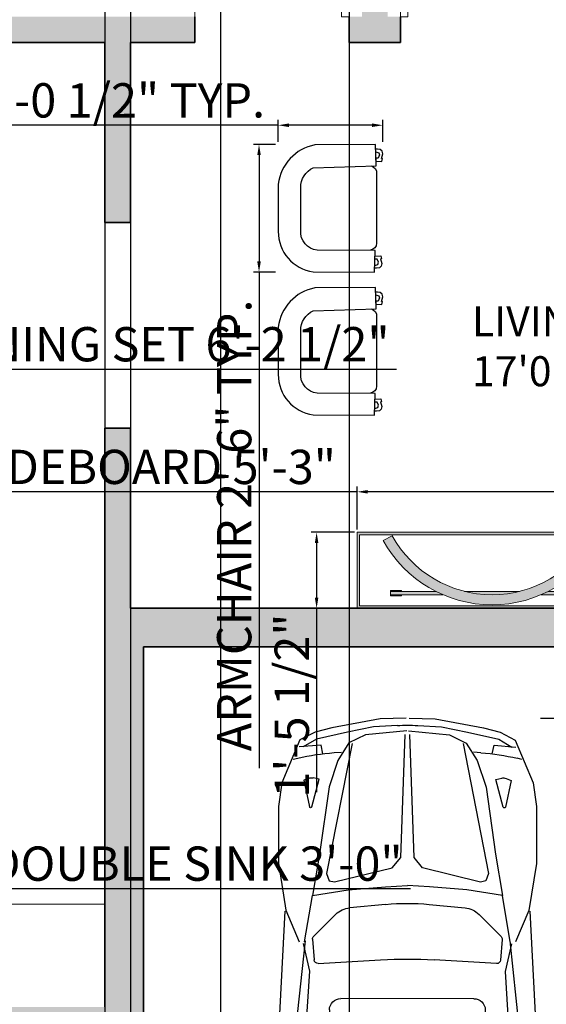
# Model space of a CAD drawing. Units: inches. Extents: x 4732 to 5926, y 2665 to 3255.
# Tile 4 of 8: x 4982 to 5104, y 2827 to 3056. Entities that reach past the tile are written whole.
import ezdxf

# ---------------------------------------------------------------- set-up
doc = ezdxf.new("R2010")
doc.units = ezdxf.units.IN
doc.layers.add('2D', color=7, linetype='Continuous')
doc.layers.add('L9012X$0', color=2, linetype='Continuous')
for name, color, linetype, lineweight in [('A-ANNO-DIMS', 2, 'Continuous', 18), ('A-AREA-IDEN', 7, 'Continuous', 18), ('A-DOOR', 3, 'Continuous', 18), ('A-FLOR-CASE', 7, 'Continuous', 18), ('A-SITE-VEHS', 8, 'Continuous', 13), ('A-WALL', 7, 'Continuous', 35), ('A-WALL-PATT', 8, 'Continuous', 13), ('aparador', 36, 'Continuous', 9), ('moveis', 254, 'Continuous', 5), ('NOI THAT', 42, 'Continuous', 18)]:
    doc.layers.add(name, color=color, linetype=linetype, lineweight=lineweight)
doc.styles.get("Standard").update_dxf_attribs({"font": 'arial.ttf'})
doc.dimstyles.new('ISO-25', dxfattribs={"dimtxt": 8, "dimasz": 2.5, "dimexe": 1.25, "dimexo": 0.625, "dimtad": 1, "dimdec": 1, "dimlunit": 3, "dimtxsty": 'Standard', "dimcen": 2.5, "dimadec": 0, "dimazin": 0, "dimtfac": 1, "dimtdec": 1, "dimtmove": 0, "dimatfit": 3, "dimfxl": 1, "dimarcsym": 0})

# ---------------------------------------------------------------- blocks, each defined once
blk = doc.blocks.new('S 1')
at = {"layer": '2D'}
blk.add_lwpolyline([(4300.17, 1811.07), (4294.36, 1811.27), (4294.5, 1827.76, -0.326306), (4305.18, 1837.77), (4318.07, 1837.77, -0.372891), (4329.09, 1828.23), (4329.16, 1811.54), (4323.28, 1811.34), (4323.21, 1827.16, 0.399039), (4317.87, 1831.63), (4306.12, 1831.63, 0.288471), (4300.71, 1828.23)], format="xyb", close=True, dxfattribs=at)
for points in [[(4296.37, 1811.14), (4296.63, 1810.34), (4297.23, 1810.21), (4298.1, 1810.54), (4298.1, 1811.14), (4298.9, 1811.14), (4299.04, 1809.54), (4298.24, 1809.34), (4298.17, 1809.61), (4296.9, 1809.27), (4296.17, 1809.47), (4295.77, 1809.94), (4295.63, 1810.74), (4295.63, 1811.21)], [(4327.35, 1811.41), (4327.09, 1810.61), (4326.49, 1810.47), (4325.62, 1810.81), (4325.62, 1811.41), (4324.82, 1811.41), (4324.68, 1809.81), (4325.48, 1809.61), (4325.55, 1809.87), (4326.82, 1809.54), (4327.55, 1809.74), (4327.95, 1810.21), (4328.09, 1811.01), (4328.09, 1811.47)]]:
    blk.add_lwpolyline(points, dxfattribs=at)
blk.add_lwpolyline([(4300.24, 1812.34, 0.33845), (4302.18, 1810.94), (4321.28, 1810.94, 0.381322), (4323.15, 1812.61, -0.892406)], format="xyb", dxfattribs=at)
blk = doc.blocks.new('Aparador ORGANICA Formatto')
at = {"layer": 'aparador', "ltscale": 0.3}
h = blk.add_hatch(color=256, dxfattribs=at)
h.dxf.hatch_style = 1
h.set_gradient(color1=(118, 213, 123), color2=(52, 168, 57), one_color=1, tint=0.43, name='INVCURVED')
h.paths.add_polyline_path([(0.8, 0.45), (-0.8, 0.45), (-0.8, 0), (0.8, 0)])
h.paths.add_polyline_path([(0.785, 0.435), (0.785, 0.015), (-0.785, 0.015), (-0.785, 0.435)], flags=16)
h.paths.add_polyline_path([(0.2911, 0.3699), (0.5365, 0.3699), (0.5365, 0.3757), (0.6011, 0.3757), (0.6011, 0.3699), (0.6011, 0.3499), (0.6011, 0.3441), (0.5365, 0.3441), (0.5365, 0.3499), (0.3338, 0.3499, -0.150336), (0.6449, 0.0488), (0.5923, 0.0199, 0.208852), (0.1632, 0.3499), (-0.1632, 0.3499, 0.208852), (-0.5923, 0.0199), (-0.6449, 0.0488, -0.150336), (-0.3338, 0.3499), (-0.5365, 0.3499), (-0.5365, 0.3441), (-0.6011, 0.3441), (-0.6011, 0.3499), (-0.6011, 0.3699), (-0.6011, 0.3757), (-0.5365, 0.3757), (-0.5365, 0.3699), (-0.2911, 0.3699, -0.206106)], flags=0)
h = blk.add_hatch(color=256, dxfattribs=at)
h.dxf.hatch_style = 1
h.set_gradient(color1=(135, 92, 69), color2=(0, 0, 0), one_color=1, name='INVCURVED')
h.paths.add_polyline_path([(-0.6449, 0.0488), (-0.5923, 0.0199, -0.590888), (0.5923, 0.0199), (0.6449, 0.0488, 0.590888)])
h = blk.add_hatch(color=256, dxfattribs=at)
h.dxf.hatch_style = 1
h.set_gradient(color1=(178, 189, 189), one_color=1, tint=1, name='CYLINDER')
h.paths.add_polyline_path([(-0.5365, 0.3757), (-0.6011, 0.3757), (-0.6011, 0.3699), (-0.5365, 0.3699)])
h.paths.add_polyline_path([(-0.5365, 0.3499), (-0.6011, 0.3499), (-0.6011, 0.3441), (-0.5365, 0.3441)])
h = blk.add_hatch(color=256, dxfattribs=at)
h.dxf.hatch_style = 1
h.set_gradient(color1=(118, 213, 123), color2=(31, 101, 35), one_color=1, tint=0.26, name='INVCURVED')
h.paths.add_polyline_path([(-0.2911, 0.3699), (-0.6011, 0.3699), (-0.6011, 0.3499), (-0.3338, 0.3499, -0.015999)])
h = blk.add_hatch(color=256, dxfattribs=at)
h.dxf.hatch_style = 1
h.set_gradient(color1=(118, 213, 123), color2=(31, 101, 35), one_color=1, tint=0.26, name='INVCURVED')
h.paths.add_polyline_path([(-0.1632, 0.3499), (0.1632, 0.3499, 0.122516)])
h = blk.add_hatch(color=256, dxfattribs=at)
h.dxf.hatch_style = 1
h.set_gradient(color1=(118, 213, 123), color2=(31, 101, 35), one_color=1, tint=0.26, name='INVCURVED')
h.paths.add_polyline_path([(0.6011, 0.3699), (0.2911, 0.3699, -0.015999), (0.3338, 0.3499), (0.6011, 0.3499)])
h = blk.add_hatch(color=256, dxfattribs=at)
h.dxf.hatch_style = 1
h.set_gradient(color1=(178, 189, 189), one_color=1, tint=1, name='CYLINDER')
h.paths.add_polyline_path([(0.6011, 0.3757), (0.5365, 0.3757), (0.5365, 0.3699), (0.6011, 0.3699)])
h.paths.add_polyline_path([(0.6011, 0.3499), (0.5365, 0.3499), (0.5365, 0.3441), (0.6011, 0.3441)])
for p, q in [((-0.5923, 0.0199), (-0.6449, 0.0488)), ((0.5923, 0.0199), (0.6449, 0.0488))]:
    blk.add_line(p, q, dxfattribs=at)
for points in [[(-0.6011, 0.3699), (-0.6011, 0.3757), (-0.5365, 0.3757), (-0.5365, 0.3699)], [(0.6011, 0.3699), (0.6011, 0.3757), (0.5365, 0.3757), (0.5365, 0.3699)], [(-0.5365, 0.3499), (-0.5365, 0.3441), (-0.6011, 0.3441), (-0.6011, 0.3499)], [(0.5365, 0.3499), (0.5365, 0.3441), (0.6011, 0.3441), (0.6011, 0.3499)]]:
    blk.add_lwpolyline(points, dxfattribs=at)
for radius in [0.7362, 0.6762]:
    blk.add_arc((0, -0.3063), radius, 28.84335, 151.15665, dxfattribs=at)
at = {"layer": 'moveis', "ltscale": 0.3}
for p, q in [((-0.6011, 0.3699), (-0.6011, 0.3499)), ((-0.2911, 0.3699), (-0.6011, 0.3699)), ((0.2911, 0.3699), (0.6011, 0.3699)), ((0.6011, 0.3699), (0.6011, 0.3499)), ((-0.6011, 0.3499), (-0.3338, 0.3499)), ((-0.1632, 0.3499), (0.1632, 0.3499)), ((0.6011, 0.3499), (0.3338, 0.3499))]:
    blk.add_line(p, q, dxfattribs=at)
for points in [[(-0.8, 0), (0.8, 0), (0.8, 0.45), (-0.8, 0.45)], [(-0.785, 0.015), (0.785, 0.015), (0.785, 0.435), (-0.785, 0.435)]]:
    blk.add_lwpolyline(points, close=True, dxfattribs=at)
blk = doc.blocks.new('*U20')
for p, q in [((0, 0), (0, -6)), ((36, 0), (36, -6))]:
    blk.add_line(p, q)
blk.add_lwpolyline([(0, 0), (0, 36), (1.75, 36), (1.75, 0)], close=True)
blk.add_arc((0, 0), 36, 0, 90)
blk = doc.blocks.new('A1099DC')
at = {"color": 0, "linetype": 'ByBlock'}
for p, q in [((1279.298465, 804.448389), (2201.430588, 851.890505)), ((2602.736326, 846.078152), (3356.693814, 785.353187)), ((272.228253, 749.073842), (265.114727, 718.465169)), ((1475.52921, 670.226262), (2282.402739, 758.004075)), ((2519.280414, 756.817792), (3387.476361, 653.818028)), ((2851.341839, 715.213377), (3126.60716, 755.701993)), ((3488.458929, 772.663345), (3732.658862, 759.86454)), ((139.051458, 595.027331), (190.951238, 683.213377)), ((179.200345, 564.515703), (190.951238, 709.631982)), ((398.733388, 644.315148), (411.280494, 678.748261)), ((411.280494, 678.748261), (588.616917, 641.417897)), ((1482.852352, 674.283145), (1175.286956, 622.180789)), ((1494.603245, 682.841284), (1678.210958, 641.166865)), ((1678.210958, 641.166865), (2462.684993, 690.847736)), ((2656.476214, 692.831247), (3376.704709, 662.004075)), ((3376.704709, 662.004075), (3510.708679, 626.736433)), ((3909.27561, 688.812956), (3837.725727, 693.401722)), ((3867.794139, 700.329656), (3900.059395, 686.767505)), ((3921.162781, 527.618662), (3921.162781, 676.138994)), ((3925.383812, 676.122818), (3955.306409, 663.545364)), ((92.537504, 388.14361), (139.051458, 595.027331)), ((405.405047, 577.538958), (396.874865, 615.894428)), ((589.014326, 626.599587), (405.405047, 577.538958)), ((1300.814287, 466.658131), (1445.712032, 613.104998)), ((1465.665584, 620.56924), (1602.893878, 610.287296)), ((236.043912, 551.980927), (179.200345, 564.515703)), ((1626.354615, 583.507504), (1602.652901, 169.222264)), ((1933.148906, 509.557888), (2330.980062, 522.200075)), ((3704.596898, 536.993674), (3795.675135, 473.385795)), ((229.117398, 477.634662), (225.714299, 427.957563)), ((3493.960271, 465.734554), (3507.923021, 209.166865)), ((3522.252709, 492.345257), (3666.066199, 475.644444)), ((3841.786866, 503.451367), (3910.58243, 515.096797)), ((3901.001848, 514.780764), (3957.150905, 375.772812)), ((1860.238743, -448.635916), (1859.369151, 433.397797)), ((2409.60024, 445.938054), (2410.49349, -460.09121)), ((3753.293176, 397.789551), (3815.226005, 132.124765)), ((3839.396146, 426.841284), (3888.358202, 417.538958)), ((3888.358202, 417.538958), (3983.199613, 359.957848)), ((57.774444, 216.608726), (92.537504, 388.14361)), ((1235.045743, 136.116317), (1257.419842, 373.755108)), ((3857.610793, 379.525702), (3912.067615, 118.157673)), ((3983.199613, 359.957848), (4035.448301, 43.94997)), ((49.168662, 58.00681), (57.774444, 216.608726)), ((3507.923021, 209.166865), (3507.64153, -4.333678)), ((4019.086894, 150.376168), (4084.69605, 122.469191)), ((4084.69605, 122.469191), (4109.177079, 60.329656)), ((4109.177079, 60.329656), (4113.094043, -5.158716)), ((3508.347273, -221.154823), (3507.644805, -7.65525)), ((3983.920268, -371.008369), (4035.545755, -54.898082)), ((4109.306686, -71.132359), (4113.094514, -5.636391)), ((49.301278, -76.507426), (58.219773, -235.092064)), ((3858.370276, -390.823819), (3912.311631, -129.348921)), ((4084.948231, -133.320044), (4109.306686, -71.132359)), ((1235.330373, -152.586046), (1258.173002, -390.180259)), ((1627.520644, -599.204785), (1603.002095, -184.967086)), ((3754.088875, -409.293325), (3815.497749, -143.506937)), ((4019.394229, -161.356334), (4084.948231, -133.320044)), ((58.219773, -235.092064), (93.320996, -406.558069)), ((3494.890446, -477.749545), (3508.347273, -221.154823)), ((3889.19258, -428.776374), (3983.920268, -371.008369)), ((3902.027941, -525.993061), (3957.902795, -386.874665)), ((93.320996, -406.558069), (140.24279, -613.349673)), ((230.077082, -495.779641), (226.576036, -446.109349)), ((3840.248961, -438.175225), (3889.19258, -428.776374)), ((1301.750547, -482.997536), (1446.936772, -629.158411)), ((3523.2353, -504.304409), (3667.01558, -487.320059)), ((3705.667171, -548.593196), (3796.61981, -484.805853)), ((3842.790735, -514.780444), (3911.609128, -526.290202)), ((237.150178, -570.112104), (180.331436, -582.758939)), ((180.331436, -582.758939), (192.368445, -727.851766)), ((1934.168526, -524.650381), (2332.023837, -536.508105)), ((3922.214148, -538.79118), (3922.506998, -687.311224)), ((140.24279, -613.349673), (192.316354, -701.433212)), ((406.561378, -595.336142), (398.106841, -633.708356)), ((590.267037, -644.034637), (406.561378, -595.336142)), ((1484.19765, -690.263206), (1176.530118, -638.767405)), ((1466.905004, -636.583294), (1604.112757, -626.030785)), ((3378.022114, -674.249887), (3511.956283, -638.718087)), ((400.0214, -662.125356), (412.636377, -696.533662)), ((412.636377, -696.533662), (589.898847, -658.853701)), ((1476.866524, -686.22077), (2283.911563, -772.40743)), ((1495.965396, -698.798158), (1679.490579, -656.761786)), ((1679.490579, -656.761786), (2464.061049, -704.895745)), ((2520.786439, -770.754078), (3388.777604, -666.042617)), ((2657.855804, -706.497136), (3378.022114, -674.249887)), ((3910.644841, -700.0086), (3839.104145, -704.738438)), ((3869.186159, -711.60707), (3901.424611, -697.981326)), ((3926.727989, -687.286725), (3956.625729, -674.650294)), ((273.723073, -767.133288), (266.549207, -736.538701)), ((2852.765183, -728.494989), (3128.109803, -768.440762)), ((3489.994314, -784.688586), (3734.168535, -771.408296)), ((1280.900818, -820.829563), (2203.124693, -866.453338)), ((2604.418191, -859.849707), (3358.254477, -797.638217))]:
    blk.add_line(p, q, dxfattribs=at)
for points in [[(-0.000783, 0.794772), (5.385043, 172.701749), (63.649891, 493.818028), (92.537504, 603.957563), (144.437284, 705.166865), (428.417214, 824.236633), (585.095796, 846.190121), (961.406447, 846.190121), (1274.27399, 797.818028), (1482.852352, 709.631982)], [(83.345007, -3.206171), (111.32237, 268.957533), (164.563706, 379.583828), (279.999271, 453.709838), (456.549665, 511.628518), (901.254996, 574.918954), (1175.286956, 622.180789), (1137.52997, 385.548359), (1118.345181, 137.317882), (1109.829198, -8.358455)], [(168.178729, 359.003083), (1030.214866, 528.397865), (1077.798844, 510.531569), (1086.170082, 475.285426), (992.832238, 91.960378), (924.218938, 35.478085), (108.447994, 6.034416)], [(0.019119, -19.392451), (5.743899, -191.288474), (64.641806, -512.289243), (93.746535, -622.371603), (145.845778, -723.478374), (430.059935, -841.987962), (586.7815, -863.632471), (963.091723, -863.198028), (1275.863278, -814.209121), (1484.26735, -725.611974)], [(83.356858, -15.227176), (111.870816, -287.335185), (165.330179, -397.856284), (280.911681, -471.754535), (457.575935, -529.324983), (902.4055, -592.045995), (1176.530118, -638.767405), (1138.306616, -402.209884), (1118.632407, -154.017717), (1109.829198, -8.358455)], [(168.904615, -377.268451), (1031.273389, -545.270714), (1078.822046, -527.310627), (1087.123771, -492.048047), (993.030273, -108.907787), (924.305735, -52.560894), (108.478017, -24.418246)]]:
    blk.add_lwpolyline(points, dxfattribs=at)
for centre, radius, start, end in [((2358.037832, -2192.08357), 3048, 85.395244, 92.945173), ((2399.99649, 588.663508), 206.166238, 54.649181, 124.776949), ((1749.553982, 373.478072), 1524, 166.916578, 176.08111), ((3392.740754, -1053.630025), 1828.8, 86.999806, 98.367602), ((3718.678317, 475.802507), 284.405862, 57.329946, 87.182375), ((2578.271641, -1134.295865), 1828.8, 87.549126, 93.623712), ((4191.049821, 605.937201), 363.988953, 166.096081, 196.353514), ((3908.462781, 676.138994), 12.7, 0, 86.330429), ((3896.252417, 523.051998), 152.4, 46.38363, 67.20138), ((446.46332, 626.922805), 50.8, 159.97873, 192.538409), ((587.047263, 633.961317), 7.62, 284.960009, 78.112462), ((1463.767788, 595.240237), 25.4, 85.715073, 135.304647), ((1600.996082, 584.958293), 25.4, 356.725615, 85.715073), ((3355.555414, 37.211519), 609.6, 55.070043, 75.255062), ((3320.85101, 50.338397), 847.430844, 356.245089, 44.519453), ((3700.933354, 318.064082), 435.542335, 30.457681, 46.38363), ((2333.400307, 446.03852), 76.2, 359.924458, 91.82012), ((3908.462781, 527.618662), 12.7, 279.607718, 0), ((3204.184594, 25.950693), 1011.814461, 358.069446, 30.457681), ((1409.148822, 359.469565), 152.4, 135.304647, 174.62136), ((1935.569151, 433.396333), 76.2, 91.82012, 179.9989), ((3519.322741, 467.114813), 25.4, 83.37601, 183.115039), ((3654.346327, 374.722669), 101.6, 13.122645, 83.37601), ((3708.414764, 348.440256), 152.4, 11.769371, 55.070043), ((2752.335538, -6.739118), 1524, 174.62136, 185.491615), ((4645.676894, -4.872483), 3048, 176.725615, 183.38736), ((3221.54491, -6.276527), 609.6, 346.99033, 13.122645), ((3315.283499, -6.18411), 609.6, 348.343604, 11.769371), ((1266.577845, -8.050136), 1219.2, 176.894161, 183.218814), ((3734.73098, -5.770579), 304.8, 350.724636, 9.388339), ((3320.962449, -62.69553), 847.430844, 315.593523, 3.867886), ((3204.248172, -38.537915), 1011.814461, 329.655294, 2.043529), ((1409.873518, -375.595566), 152.4, 185.491615, 224.808328), ((3709.113243, -360.032616), 152.4, 305.042932, 348.343604), ((1936.438592, -448.484202), 76.2, 180.114076, 268.292856), ((3655.096735, -386.42159), 101.6, 276.736965, 346.99033), ((1750.305335, -388.625277), 1524, 184.031865, 193.196397), ((2334.293902, -460.341926), 76.2, 268.292856, 0.188517), ((3520.255588, -479.079792), 25.4, 176.997936, 276.736965), ((4192.255091, -616.577407), 363.988953, 163.759461, 194.016894), ((3355.640902, -49.500248), 609.6, 284.857913, 305.042932), ((3909.514173, -538.816222), 12.7, 0.112975, 80.505257), ((3701.571953, -329.671253), 435.542335, 313.729345, 329.655294), ((447.716945, -644.638934), 50.8, 167.574566, 200.134245), ((588.314493, -651.400231), 7.62, 282.000513, 75.152966), ((1464.957267, -611.258083), 25.4, 224.808328, 274.397903), ((1602.165021, -600.705574), 25.4, 274.397903, 3.38736), ((3897.294828, -534.273643), 152.4, 292.911596, 313.729345), ((2576.048678, 1120.472221), 1828.8, 266.489263, 272.563849), ((3909.807023, -687.336265), 12.7, 273.782546, 0.112975), ((2401.171182, -602.835323), 206.166238, 235.336026, 305.463794), ((3390.675263, 1041.412497), 1828.8, 261.745373, 273.113169), ((3719.627907, -487.374382), 284.405862, 272.930601, 302.78303), ((2353.729565, 2177.823616), 3048, 267.167802, 274.717731)]:
    blk.add_arc(centre, radius, start, end, dxfattribs=at)
blk = doc.blocks.new('VI')
at = {"layer": 'L9012X$0'}
blk.add_blockref('A1099DC', (0, 0), dxfattribs=at)
blk = doc.blocks.new('COUNTER-KITCHEN-L')
for p, q in [((0, 48), (24, 48)), ((24, 0), (24, 48)), ((24, 0), (120, 0))]:
    blk.add_line(p, q)
blk = doc.blocks.new('*D78')
at = {"layer": 'A-ANNO-DIMS', "color": 0, "lineweight": -2, "transparency": 16777216}
for p, q in [((5041.22, 3027.15), (5036.12, 3027.15)), ((5037.37, 3024.65), (5037.37, 2999.85)), ((5041.22, 2997.35), (5036.12, 2997.35)), ((5037.37, 2997.35), (5037.37, 2881.66))]:
    blk.add_line(p, q, dxfattribs=at)
at = {"layer": 'A-ANNO-DIMS', "color": 0, "transparency": 16777216}
for points in [[(5036.96, 3024.65), (5037.79, 3024.65), (5037.37, 3027.15)], [(5036.96, 2999.85), (5037.79, 2999.85), (5037.37, 2997.35)]]:
    blk.add_solid(points, dxfattribs=at)
at = {"layer": 'Defpoints', "color": 0, "transparency": 16777216}
for p in [(5041.84, 3027.15), (5037.37, 2997.35), (5041.84, 2997.35)]:
    blk.add_point(p, dxfattribs=at)
at = {"layer": 'A-ANNO-DIMS', "color": 0, "transparency": 16777216, "insert": (5032.61, 2938.26), "char_height": 8, "attachment_point": 5, "rotation": 90}
blk.add_mtext('ARMCHAIR 2\'-6" TYP.', dxfattribs=at)
blk = doc.blocks.new('*D79')
at = {"layer": 'A-ANNO-DIMS', "color": 0, "lineweight": -2, "transparency": 16777216}
for p, q in [((5041.84, 3027.77), (5041.84, 3032.86)), ((5066.25, 3027.77), (5066.25, 3032.86)), ((5041.84, 3031.61), (4970.55, 3031.61)), ((5063.75, 3031.61), (5044.34, 3031.61))]:
    blk.add_line(p, q, dxfattribs=at)
at = {"layer": 'A-ANNO-DIMS', "color": 0, "transparency": 16777216}
for points in [[(5044.34, 3032.03), (5044.34, 3031.2), (5041.84, 3031.61)], [(5063.75, 3032.03), (5063.75, 3031.2), (5066.25, 3031.61)]]:
    blk.add_solid(points, dxfattribs=at)
at = {"layer": 'Defpoints', "color": 0, "transparency": 16777216}
for p in [(5041.84, 3031.61), (5041.84, 3027.15), (5066.25, 3027.15)]:
    blk.add_point(p, dxfattribs=at)
at = {"layer": 'A-ANNO-DIMS', "color": 0, "transparency": 16777216, "insert": (5004.95, 3036.38), "char_height": 8, "attachment_point": 5}
blk.add_mtext('2\'-0 1/2" TYP.', dxfattribs=at)
blk = doc.blocks.new('*D84')
at = {"layer": 'A-ANNO-DIMS', "color": 0, "lineweight": -2, "transparency": 16777216}
for p, q in [((4933.87, 2848.78), (4933.87, 2854.8)), ((4936.37, 2853.55), (4967.37, 2853.55)), ((4969.87, 2848.78), (4969.87, 2854.8)), ((4969.87, 2853.55), (5072.74, 2853.55))]:
    blk.add_line(p, q, dxfattribs=at)
at = {"layer": 'A-ANNO-DIMS', "color": 0, "transparency": 16777216}
for points in [[(4936.37, 2853.97), (4936.37, 2853.14), (4933.87, 2853.55)], [(4967.37, 2853.97), (4967.37, 2853.14), (4969.87, 2853.55)]]:
    blk.add_solid(points, dxfattribs=at)
at = {"layer": 'Defpoints', "color": 0, "transparency": 16777216}
for p in [(4969.87, 2853.55), (4933.87, 2848.15), (4969.87, 2848.15)]:
    blk.add_point(p, dxfattribs=at)
at = {"layer": 'A-ANNO-DIMS', "color": 0, "transparency": 16777216, "insert": (5022.55, 2858.32), "char_height": 8, "attachment_point": 5}
blk.add_mtext('DOUBLE SINK 3\'-0"', dxfattribs=at)
blk = doc.blocks.new('*D88')
at = {"layer": 'A-ANNO-DIMS', "color": 0, "lineweight": -2, "transparency": 16777216}
for p, q in [((4884.65, 2985.28), (4884.65, 2973.48)), ((4959.16, 2985.28), (4959.16, 2973.48)), ((4887.15, 2974.73), (4956.66, 2974.73)), ((4959.16, 2974.73), (5069.48, 2974.73))]:
    blk.add_line(p, q, dxfattribs=at)
at = {"layer": 'A-ANNO-DIMS', "color": 0, "transparency": 16777216}
for points in [[(4887.15, 2975.15), (4887.15, 2974.31), (4884.65, 2974.73)], [(4956.66, 2975.15), (4956.66, 2974.31), (4959.16, 2974.73)]]:
    blk.add_solid(points, dxfattribs=at)
at = {"layer": 'Defpoints', "color": 0, "transparency": 16777216}
for p in [(4884.65, 2985.91), (4959.16, 2985.91), (4959.16, 2974.73)]:
    blk.add_point(p, dxfattribs=at)
at = {"layer": 'A-ANNO-DIMS', "color": 0, "transparency": 16777216, "insert": (5015.57, 2979.49), "char_height": 8, "attachment_point": 5}
blk.add_mtext('DINING SET 6\'-2 1/2"', dxfattribs=at)
blk = doc.blocks.new('*D94')
at = {"layer": 'A-ANNO-DIMS', "color": 0, "lineweight": -2, "transparency": 16777216}
for p, q in [((5060.26, 2937.27), (5060.26, 2947.35)), ((5123.25, 2937.27), (5123.25, 2947.35)), ((5060.26, 2946.1), (4966.35, 2946.1)), ((5120.75, 2946.1), (5062.76, 2946.1))]:
    blk.add_line(p, q, dxfattribs=at)
at = {"layer": 'A-ANNO-DIMS', "color": 0, "transparency": 16777216}
for points in [[(5062.76, 2946.52), (5062.76, 2945.68), (5060.26, 2946.1)], [(5120.75, 2946.52), (5120.75, 2945.68), (5123.25, 2946.1)]]:
    blk.add_solid(points, dxfattribs=at)
at = {"layer": 'Defpoints', "color": 0, "transparency": 16777216}
for p in [(5060.26, 2946.1), (5060.26, 2936.65), (5123.25, 2936.65)]:
    blk.add_point(p, dxfattribs=at)
at = {"layer": 'A-ANNO-DIMS', "color": 0, "transparency": 16777216, "insert": (5012.05, 2950.87), "char_height": 8, "attachment_point": 5}
blk.add_mtext('SIDEBOARD 5\'-3"', dxfattribs=at)
blk = doc.blocks.new('*D95')
at = {"layer": 'A-ANNO-DIMS', "color": 0, "lineweight": -2, "transparency": 16777216}
for p, q in [((5059.63, 2936.65), (5049.56, 2936.65)), ((5050.81, 2934.15), (5050.81, 2921.43)), ((5059.63, 2918.93), (5049.56, 2918.93)), ((5050.81, 2918.93), (5050.81, 2876.03))]:
    blk.add_line(p, q, dxfattribs=at)
at = {"layer": 'A-ANNO-DIMS', "color": 0, "transparency": 16777216}
for points in [[(5050.39, 2934.15), (5051.22, 2934.15), (5050.81, 2936.65)], [(5050.39, 2921.43), (5051.22, 2921.43), (5050.81, 2918.93)]]:
    blk.add_solid(points, dxfattribs=at)
at = {"layer": 'Defpoints', "color": 0, "transparency": 16777216}
for p in [(5060.26, 2936.65), (5050.81, 2918.93), (5060.26, 2918.93)]:
    blk.add_point(p, dxfattribs=at)
at = {"layer": 'A-ANNO-DIMS', "color": 0, "transparency": 16777216, "insert": (5046.05, 2896.23), "char_height": 8, "attachment_point": 5, "rotation": 90}
blk.add_mtext('1\'-5 1/2"', dxfattribs=at)
blk = doc.blocks.new('*D96')
at = {"layer": 'A-ANNO-DIMS', "color": 0, "lineweight": -2, "transparency": 16777216}
for p, q in [((5103.06, 2893.31), (5125.97, 2893.31)), ((5124.72, 2890.81), (5124.72, 2747.23)), ((5103.06, 2744.73), (5125.97, 2744.73))]:
    blk.add_line(p, q, dxfattribs=at)
at = {"layer": 'A-ANNO-DIMS', "color": 0, "transparency": 16777216}
for points in [[(5124.3, 2890.81), (5125.14, 2890.81), (5124.72, 2893.31)], [(5124.3, 2747.23), (5125.14, 2747.23), (5124.72, 2744.73)]]:
    blk.add_solid(points, dxfattribs=at)
at = {"layer": 'Defpoints', "color": 0, "transparency": 16777216}
for p in [(5102.43, 2893.31), (5102.43, 2744.73), (5124.72, 2744.73)]:
    blk.add_point(p, dxfattribs=at)
at = {"layer": 'A-ANNO-DIMS', "color": 0, "transparency": 16777216, "insert": (5119.96, 2819.02), "char_height": 8, "attachment_point": 5, "rotation": 90}
blk.add_mtext('CAR 12\'-4 1/2"', dxfattribs=at)
blk = doc.blocks.new('*D107')
at = {"layer": 'A-ANNO-DIMS', "color": 0, "lineweight": -2, "transparency": 16777216}
for p, q in [((5028.38, 3098.31), (5028.38, 2665.12)), ((5058.38, 3098.31), (5058.38, 2665.12)), ((5030.88, 2666.37), (5055.88, 2666.37))]:
    blk.add_line(p, q, dxfattribs=at)
at = {"layer": 'A-ANNO-DIMS', "color": 0, "transparency": 16777216}
for points in [[(5030.88, 2666.79), (5030.88, 2665.96), (5028.38, 2666.37)], [(5055.88, 2666.79), (5055.88, 2665.96), (5058.38, 2666.37)]]:
    blk.add_solid(points, dxfattribs=at)
at = {"layer": 'Defpoints', "color": 0, "transparency": 16777216}
for p in [(5028.38, 3098.93), (5058.38, 3098.93), (5058.38, 2666.37)]:
    blk.add_point(p, dxfattribs=at)
at = {"layer": 'A-ANNO-DIMS', "color": 0, "transparency": 16777216, "insert": (5043.38, 2671.08), "char_height": 8, "attachment_point": 5}
blk.add_mtext('2\'-6"', dxfattribs=at)
blk = doc.blocks.new('*D114')
at = {"layer": 'A-ANNO-DIMS', "color": 0, "lineweight": -2, "transparency": 16777216}
for p, q in [((5007.38, 3104.31), (5007.38, 2665.12)), ((5001.38, 3098.31), (5001.38, 2665.12)), ((4998.88, 2666.37), (4996.38, 2666.37)), ((5001.38, 2666.37), (5007.38, 2666.37)), ((5009.88, 2666.37), (5034.9, 2666.37))]:
    blk.add_line(p, q, dxfattribs=at)
at = {"layer": 'A-ANNO-DIMS', "color": 0, "transparency": 16777216}
for points in [[(4998.88, 2666.79), (4998.88, 2665.96), (5001.38, 2666.37)], [(5009.88, 2666.79), (5009.88, 2665.96), (5007.38, 2666.37)]]:
    blk.add_solid(points, dxfattribs=at)
at = {"layer": 'Defpoints', "color": 0, "transparency": 16777216}
for p in [(5007.38, 3104.93), (5001.38, 3098.93), (5007.38, 2666.37)]:
    blk.add_point(p, dxfattribs=at)
at = {"layer": 'A-ANNO-DIMS', "color": 0, "transparency": 16777216, "insert": (5023.64, 2671.08), "char_height": 8, "attachment_point": 5}
blk.add_mtext('0\'-6"', dxfattribs=at)

msp = doc.modelspace()

# ---------------------------------------------------------------- hatches: boundary and pattern name
at = {"layer": 'A-WALL-PATT'}
h = msp.add_hatch(color=256, dxfattribs=at)
h.dxf.hatch_style = 1
h.paths.add_polyline_path([(4905.38, 3185.93), (4848.38, 3185.93), (4848.38, 3146.93), (4857.38, 3146.93), (4857.38, 3176.93), (4905.38, 3176.93)])
h.paths.add_polyline_path([(5022.38, 3185.93), (4953.38, 3185.93), (4953.38, 3176.93), (4966.1, 3176.93), (5001.38, 3176.93), (5001.38, 3098.93), (5028.38, 3098.93), (5028.38, 3104.93), (5007.38, 3104.93), (5007.38, 3176.93), (5022.38, 3176.93)])
h.paths.add_polyline_path([(5115.38, 3185.93), (5046.38, 3185.93), (5046.38, 3176.93), (5061.38, 3176.93), (5061.38, 3104.93), (5058.38, 3104.93), (5058.38, 3098.93), (5067.38, 3098.93), (5067.38, 3176.93), (5115.38, 3176.93)])
h.paths.add_polyline_path([(5220.38, 3185.93), (5163.38, 3185.93), (5163.38, 3176.93), (5168.97, 3176.93), (5211.38, 3176.93), (5211.38, 3146.93), (5220.38, 3146.93)])
h.paths.add_polyline_path([(4857.38, 3086.93), (4848.38, 3086.93), (4848.38, 3026.93), (4857.38, 3026.93), (4857.38, 3050.93), (5001.38, 3050.93), (5001.38, 3008.93), (5007.38, 3008.93), (5007.38, 3050.93), (5022.38, 3050.93), (5022.38, 3056.93), (4857.38, 3056.93)])
h.paths.add_polyline_path([(4857.38, 2978.93), (4848.38, 2978.93), (4848.38, 2945.93), (4872.38, 2945.93), (4872.38, 2933.93), (4875.38, 2933.93), (4881.38, 2933.93), (4881.38, 2954.93), (4857.38, 2954.93)])
h.paths.add_polyline_path([(4881.38, 2903.93), (4875.38, 2903.93), (4872.38, 2903.93), (4872.38, 2897.93), (4881.38, 2897.93)])
h.paths.add_polyline_path([(4881.38, 2849.93), (4872.38, 2849.93), (4872.38, 2828.75), (4872.38, 2825.93), (4848.38, 2825.93), (4848.38, 2804.93), (4857.38, 2804.93), (4857.38, 2816.93), (4929.38, 2816.93), (4929.38, 2825.93), (4881.38, 2825.93)])
h.paths.add_polyline_path([(4975.38, 2744.93), (4857.38, 2744.93), (4857.38, 2756.93), (4848.38, 2756.93), (4848.38, 2735.93), (4975.38, 2735.93)])
h.paths.add_polyline_path([(5160.38, 2915.93), (5160.38, 2918.93), (5007.38, 2918.93), (5007.38, 2960.93), (5001.38, 2960.93), (5001.38, 2825.93), (4977.38, 2825.93), (4977.38, 2816.93), (5010.38, 2816.93), (5010.38, 2909.93), (5160.38, 2909.93)])
h.paths.add_polyline_path([(5220.38, 2948.93), (5211.38, 2948.93), (5211.38, 2918.93), (5208.38, 2918.93), (5208.38, 2909.93), (5220.38, 2909.93)])
h.paths.add_polyline_path([(5220.38, 3086.93), (5211.38, 3086.93), (5211.38, 3056.93), (5106.38, 3056.93), (5106.38, 3050.93), (5211.38, 3050.93), (5211.38, 3020.93), (5220.38, 3020.93)])
h.paths.add_polyline_path([(5067.38, 3098.93), (5061.38, 3098.93), (5061.38, 3056.93), (5058.38, 3056.93), (5058.38, 3050.93), (5061.38, 3050.93), (5070.38, 3050.93), (5070.38, 3056.93), (5067.38, 3056.93)])
h.paths.add_polyline_path([(4883.76, 2941.13), (4938.24, 2941.13), (4938.24, 2949.38), (4883.76, 2949.38)], flags=9)
h.paths.add_polyline_path([(4840.48, 3026.79), (4840.48, 3093.88), (4825.54, 3093.88), (4825.54, 3026.79)], flags=9)
h.paths.add_polyline_path([(5245.66, 2994.98), (5245.66, 3062.07), (5230.72, 3062.07), (5230.72, 2994.98)], flags=9)
h.paths.add_polyline_path([(4994.89, 3193.24), (5061.99, 3193.24), (5061.99, 3208.18), (4994.89, 3208.18)], flags=9)
h.paths.add_polyline_path([(5081.53, 3115.35), (5081.53, 3161.13), (5073.28, 3161.13), (5073.28, 3115.35)], flags=25)
h.paths.add_polyline_path([(4997.53, 3115.35), (4997.53, 3161.13), (4989.28, 3161.13), (4989.28, 3115.35)], flags=25)
h.paths.add_polyline_path([(5175.31, 2866.04), (5202.42, 2866.04), (5202.42, 2876.71), (5175.31, 2876.71)], flags=9)
h.paths.add_polyline_path([(4820.13, 2876.28), (4869.1, 2876.28), (4869.1, 2902.89), (4820.13, 2902.89)], flags=9)
h.paths.add_polyline_path([(5104.69, 2868.81), (5158.82, 2868.81), (5158.82, 2895.42), (5104.69, 2895.42)], flags=25)
h.paths.add_polyline_path([(5084.11, 2966.75), (5138.25, 2966.75), (5138.25, 2993.36), (5084.11, 2993.36)], flags=9)
h.paths.add_polyline_path([(4897.84, 3000.24), (4946.81, 3000.24), (4946.81, 3026.85), (4897.84, 3026.85)], flags=9)
h.paths.add_polyline_path([(5009.53, 3133.48), (5059.32, 3133.48), (5059.32, 3160.09), (5009.53, 3160.09)], flags=9)
h.paths.add_polyline_path([(5124.24, 3088.37), (5180.47, 3088.37), (5180.47, 3114.99), (5124.24, 3114.99)], flags=9)
h.paths.add_polyline_path([(4897.52, 3088.37), (4965.52, 3088.37), (4965.52, 3114.99), (4897.52, 3114.99)], flags=9)
h.paths.add_polyline_path([(4924.5, 2879.19), (4978.63, 2879.19), (4978.63, 2905.8), (4924.5, 2905.8)], flags=9)

# ---------------------------------------------------------------- linework, layer by layer
at = {"layer": 'A-WALL'}
for p, q in [((5022.38, 3056.93), (5022.38, 3050.93)), ((5058.38, 3056.93), (5058.38, 3050.93)), ((5070.38, 3056.93), (5070.38, 3050.93)), ((4857.38, 3050.93), (5001.38, 3050.93)), ((5001.38, 3008.93), (5001.38, 3050.93)), ((5007.38, 3050.93), (5022.38, 3050.93)), ((5007.38, 3008.93), (5007.38, 3050.93)), ((5058.38, 3050.93), (5061.38, 3050.93)), ((5061.38, 3050.93), (5070.38, 3050.93)), ((5001.38, 3008.93), (5007.38, 3008.93)), ((5001.38, 2825.93), (5001.38, 2960.93)), ((5001.38, 2960.93), (5007.38, 2960.93)), ((5007.38, 2918.93), (5007.38, 2960.93)), ((5007.38, 2918.93), (5160.38, 2918.93)), ((5010.38, 2816.93), (5010.38, 2909.93)), ((5010.38, 2909.93), (5160.38, 2909.93))]:
    msp.add_line(p, q, dxfattribs=at)

# ---------------------------------------------------------------- block references
at = {"layer": 'A-DOOR', "xscale": -1}
msp.add_blockref('*U20', (5058.38, 3056.93), dxfattribs=at)
at = {"layer": 'A-DOOR'}
msp.add_blockref('*U20', (5070.38, 3056.93), dxfattribs=at)
at = {"layer": 'A-FLOR-CASE'}
msp.add_blockref('COUNTER-KITCHEN-L', (4881.38, 2849.93), dxfattribs=at)
at = {"layer": 'A-SITE-VEHS', "xscale": -0.0351896714874634, "yscale": 0.0351896714874634, "zscale": 0.0351896714874634, "rotation": 90}
msp.add_blockref('VI', (5071.71, 2893.31), dxfattribs=at)
at = {"layer": 'NOI THAT'}
for name, p, xscale, yscale, zscale, rotation in [('S 1', (6615.55, 6704.46), -0.8563117011609614, 0.8563117011609614, 0.8563117011609614, 90), ('S 1', (6615.55, 6671.1), -0.8563117011609614, 0.8563117011609614, 0.8563117011609614, 90), ('Aparador ORGANICA Formatto', (5091.75, 2936.65), 39.3701, 39.3701, 39.3701, 180)]:
    msp.add_blockref(name, p, dxfattribs=dict(at, xscale=xscale, yscale=yscale, zscale=zscale, rotation=rotation))

# ---------------------------------------------------------------- texts
at = {"layer": 'A-AREA-IDEN', "insert": (5087.07, 2989.4), "char_height": 7, "attachment_point": 1}
msp.add_mtext_dynamic_manual_height_columns('{\\fTimes New Roman|b0|i0|c0|p18;LIVING 17\'0"X11\'0"}', width=61.0557, gutter_width=12.5, heights=[0], dxfattribs=at)

# ---------------------------------------------------------------- dimensions: what is measured, and where the dimension line sits
at = {"layer": 'A-ANNO-DIMS'}
for base, p1, p2, picture, middle in [((5007.38, 2666.37), (5001.38, 3098.93), (5007.38, 3104.93), '*D114', (5023.64, 2671.08)), ((5058.38, 2666.37), (5028.38, 3098.93), (5058.38, 3098.93), '*D107', (5043.38, 2671.08))]:
    dim = msp.add_linear_dim(base=base, p1=p1, p2=p2, dimstyle='ISO-25', override={"dimdec": 1, "dimlfac": 1, "dimrnd": 0, "dimzin": 1, "dimdsep": 46, "dimlunit": 4, "dimfrac": 2}, dxfattribs=at)
    dim.commit()
    dim.dimension.update_dxf_attribs({"geometry": picture, "text_midpoint": middle})
for base, p1, p2, angle, text, picture, middle in [((5041.84, 3031.61), (5066.25, 3027.15), (5041.84, 3027.15), 180, '<> TYP.', '*D79', (5004.95, 3036.38)), ((5037.37, 2997.35), (5041.84, 3027.15), (5041.84, 2997.35), 270, 'ARMCHAIR <> TYP.', '*D78', (5032.61, 2938.26)), ((5060.26, 2946.1), (5123.25, 2936.65), (5060.26, 2936.65), 180, 'SIDEBOARD <>', '*D94', (5012.05, 2950.87)), ((5124.72, 2744.73), (5102.43, 2893.31), (5102.43, 2744.73), 270, 'CAR <>', '*D96', (5119.96, 2819.02))]:
    dim = msp.add_linear_dim(base=base, p1=p1, p2=p2, angle=angle, text=text, dimstyle='ISO-25', override={"dimdec": 1, "dimlfac": 1, "dimrnd": 0, "dimzin": 1, "dimdsep": 46, "dimlunit": 4, "dimfrac": 2}, dxfattribs=at)
    dim.commit()
    dim.dimension.update_dxf_attribs({"geometry": picture, "text_midpoint": middle})
for base, p1, p2, text, picture, middle in [((4959.16, 2974.73), (4884.65, 2985.91), (4959.16, 2985.91), 'DINING SET <>', '*D88', (5015.57, 2979.49)), ((4969.87, 2853.55), (4933.87, 2848.15), (4969.87, 2848.15), 'DOUBLE SINK <>', '*D84', (5022.55, 2858.32))]:
    dim = msp.add_linear_dim(base=base, p1=p1, p2=p2, text=text, dimstyle='ISO-25', override={"dimdec": 1, "dimlfac": 1, "dimrnd": 0, "dimzin": 1, "dimdsep": 46, "dimlunit": 4, "dimfrac": 2}, dxfattribs=at)
    dim.commit()
    dim.dimension.update_dxf_attribs({"geometry": picture, "text_midpoint": middle})
dim = msp.add_linear_dim(base=(5050.81, 2918.93), p1=(5060.26, 2936.65), p2=(5060.26, 2918.93), angle=270, dimstyle='ISO-25', override={"dimdec": 1, "dimlfac": 1, "dimrnd": 0, "dimzin": 1, "dimdsep": 46, "dimlunit": 4, "dimfrac": 2}, dxfattribs=at)
dim.commit()
dim.dimension.update_dxf_attribs({"geometry": '*D95', "text_midpoint": (5046.05, 2896.23)})

doc.saveas('drawing.dxf')
